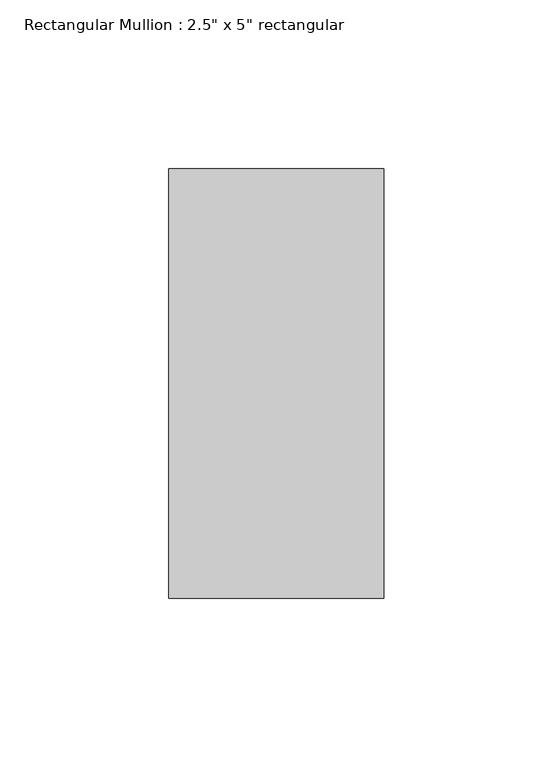
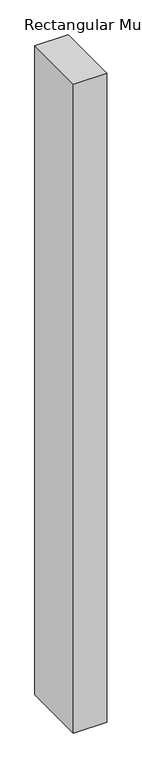
"""IFC4 building model written with IfcOpenShell, lengths in millimetres: member geometry."""

from ifc_helpers import new_model, si_unit, frame, origin, place, context, project, spatial, polyline, outline, extrude, source, transform, mapped, element, save


def member_d37749d9(model_context):
    return source(origin(), model_context, "Body", "SweptSolid", [
        extrude(outline(polyline([(0.0, 63.5), (0.0, -63.5), (-63.5, -63.5), (-63.5, 63.5), (0.0, 63.5)])), frame((0.0, 0.0, -1308.1), z_axis=(0.0, 0.0, 1.0), x_axis=(1.0, 0.0, 0.0)), (0.0, 0.0, 1.0), 1308.1),
    ])


if __name__ == "__main__":
    model = new_model("IFC4")
    model_context = context("Model", 3, world=origin())
    ifc_project = project(units=[si_unit("LENGTHUNIT", "METRE", prefix="MILLI")], contexts=[model_context])
    site = spatial("IfcSite", under=ifc_project)
    building = spatial("IfcBuilding", under=site)
    placement = place(None, origin())
    member_shape = member_d37749d9(model_context)
    element("IfcMember", 1, ObjectType="Rectangular Mullion : 2.5\" x 5\" rectangular", at=placement, inside=building, context=model_context, shape_type="MappedRepresentation", body=[
        mapped(member_shape, transform((0.0, 0.0, 0.0), x_axis=(1.0, 0.0, 0.0), y_axis=(0.0, 1.0, 0.0), z_axis=(0.0, 0.0, 1.0))),
    ])
    save(model, "model.ifc")

# Revit data of these elements
# Type "Rectangular Mullion : 2.5\" x 5\" rectangular"
#   built-in parameter 1007304 = 0.416667 (stored number, unit not read)
#   built-in parameter 1007301 = 0.104167 (stored number, unit not read)
#   built-in parameter 1007300 = 0.104167 (stored number, unit not read)
# Element 1 (IfcMember, "Rectangular Mullion : 2.5\" x 5\" rectangular")
#   Materials on its faces: "Iron, Ductile"
# Materials
#   "Iron, Ductile": class "Metal", colour RGB 0 0 0, transparency 0, Description = "Ductile cast iron", Cost = 0
